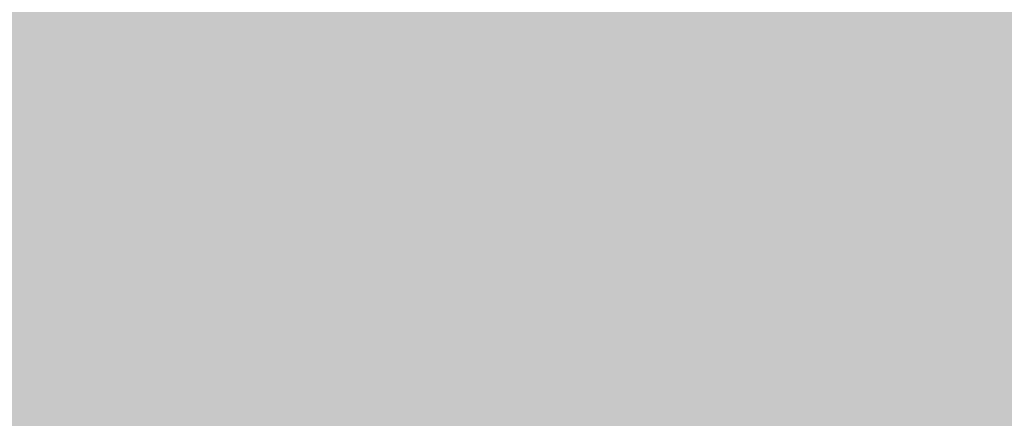
# Model space of a CAD drawing. Units: millimetres. Extents: x 0 to 2267, y 0 to 1823.
# Tile 127 of 256: x 1600.369 to 1605.705, y 1232.602 to 1234.764. Entities that reach past the tile are written whole.
import ezdxf

# ---------------------------------------------------------------- set-up
doc = ezdxf.new("R2010")
doc.units = ezdxf.units.MM
doc.header["$MEASUREMENT"] = 0
doc.layers.add('M-HATC', color=252, linetype='Continuous', lineweight=18)

msp = doc.modelspace()

# ---------------------------------------------------------------- hatches: boundary and pattern name
at = {"layer": 'M-HATC'}
h = msp.add_hatch(color=256, dxfattribs=at)
h.dxf.hatch_style = 1
h.paths.add_polyline_path([(2065.771, 1618.062, 0.236068), (2055.771, 1638.062), (1381.0868, 1638.062, 0.236068), (1371.0868, 1618.062), (1371.0868, 1603.062), (2055.771, 1603.062), (2065.771, 1603.062)])
h.paths.add_polyline_path([(2062.7718, 1550.2964), (2062.7718, 1560.2964), (1374.086, 1560.2964), (1374.086, 1550.2964), (1374.086, 1540.2964), (1384.086, 1540.2964), (1389.086, 1540.2964), (2062.7718, 1540.2964)])
h.paths.add_polyline_path([(1930.9289, 1282.7656), (1505.9289, 1282.7656), (1587.6276, 1235.5968, 0.131652), (1600.1276, 1232.2475), (1836.7302, 1232.2475, 0.131652), (1849.2302, 1235.5968)])
h.paths.add_polyline_path([(1930.9289, 1117.4171), (1905.9289, 1117.4171), (1505.9289, 1117.4171), (1505.9289, 1077.4171), (1930.9289, 1077.4171)])
h = msp.add_hatch(color=256, dxfattribs=at)
h.dxf.hatch_style = 1
h.paths.add_polyline_path([(2055.771, 1603.062), (1381.0868, 1603.062), (1381.0868, 1598.062), (2055.771, 1598.062)])
h.paths.add_polyline_path([(2055.771, 1598.062), (1381.0868, 1598.062), (1381.0868, 1593.062), (2055.771, 1593.062)])
h.paths.add_polyline_path([(2051.3074, 1536.7609), (1385.5504, 1536.7609), (1385.5504, 1526.7609), (1387.5504, 1526.7609), (1388.5366, 1525.0528), (1385.3319, 1521.2335), (1385.3319, 1521.2226), (2050.2542, 1522.7491), (2048.3212, 1525.0528), (2049.3074, 1526.7609), (2051.3074, 1526.7609)])
edge = h.paths.add_edge_path()
edge.add_arc((1847.5345, 1379.1492), 135, 222.603061, 222.890851, ccw=False)
edge.add_line((1748.1663, 1287.7656), (1683.0921, 1287.7656))
edge.add_arc((1583.7239, 1379.1492), 135, 317.109149, 317.396939, ccw=False)
edge.add_arc((1678.9686, 1290.6707), 5, 222.8909, 317.1091, ccw=False)
edge.add_arc((1774.2133, 1379.1492), 135, 222.603061, 222.890851, ccw=False)
edge.add_line((1674.8451, 1287.7656), (1609.7709, 1287.7656))
edge.add_arc((1510.4027, 1379.1492), 135, 317.109149, 317.396939, ccw=False)
edge.add_arc((1605.6474, 1290.6707), 5, 222.8909, 317.1091, ccw=False)
edge.add_arc((1700.8921, 1379.1492), 135, 222.603061, 222.890851, ccw=False)
edge.add_line((1601.5239, 1287.7656), (1536.4497, 1287.7656))
edge.add_arc((1437.0815, 1379.1492), 135, 317.109149, 317.396939, ccw=False)
edge.add_arc((1532.3262, 1290.6707), 5, 222.8909, 317.1091, ccw=False)
edge.add_arc((1627.5709, 1379.1492), 135, 222.603061, 222.890851, ccw=False)
edge.add_line((1528.2027, 1287.7656), (1505.9289, 1287.7656))
edge.add_spline(control_points=[(1505.9289, 1287.7656), (1504.2622, 1287.7656), (1504.2622, 1282.7656), (1505.9289, 1282.7656)], knot_values=[0, 0, 0, 0, 5, 5, 5, 5], degree=3, periodic=0)
edge.add_line((1505.9289, 1282.7656), (1930.9289, 1282.7656))
edge.add_spline(control_points=[(1930.9289, 1282.7656), (1932.5956, 1282.7656), (1932.5956, 1287.7656), (1930.9289, 1287.7656)], knot_values=[0, 0, 0, 0, 5, 5, 5, 5], degree=3, periodic=0)
edge.add_line((1930.9289, 1287.7656), (1903.0557, 1287.7656))
edge.add_arc((1803.6875, 1379.1492), 135, 317.109149, 317.396939, ccw=False)
edge.add_arc((1898.9322, 1290.6707), 5, 222.8909, 317.1091, ccw=False)
edge.add_arc((1994.1769, 1379.1492), 135, 222.603061, 222.890851, ccw=False)
edge.add_line((1894.8087, 1287.7656), (1829.7345, 1287.7656))
edge.add_arc((1730.3663, 1379.1492), 135, 317.109149, 317.396939, ccw=False)
edge.add_arc((1825.611, 1290.6707), 5, 222.8909, 317.1091, ccw=False)
edge.add_arc((1920.8557, 1379.1492), 135, 222.603061, 222.890851, ccw=False)
edge.add_line((1821.4875, 1287.7656), (1756.4133, 1287.7656))
edge.add_arc((1657.0451, 1379.1492), 135, 317.109149, 317.396939, ccw=False)
edge.add_arc((1752.2898, 1290.6707), 5, 222.8909, 317.1091, ccw=False)
edge = h.paths.add_edge_path()
edge.add_spline(control_points=[(1843.4289, 1227.2475), (1845.0956, 1227.2475), (1845.0956, 1232.2475), (1843.4289, 1232.2475)], knot_values=[0, 0, 0, 0, 5, 5, 5, 5], degree=3, periodic=0)
edge.add_line((1843.4289, 1232.2475), (1593.4289, 1232.2475))
edge.add_spline(control_points=[(1593.4289, 1232.2475), (1591.7622, 1232.2475), (1591.7622, 1227.2475), (1593.4289, 1227.2475)], knot_values=[0, 0, 0, 0, 5, 5, 5, 5], degree=3, periodic=0)
edge.add_line((1593.4289, 1227.2475), (1843.4289, 1227.2475))
h.paths.add_polyline_path([(1905.9289, 1127.4171), (1530.9289, 1127.4171, 0.414214), (1520.9289, 1117.4171), (1530.9289, 1117.4171), (1915.9289, 1117.4171, 0.414214)])
edge = h.paths.add_edge_path()
edge.add_arc((1397.0858, 1498.4078), 12.7299, 90.78215, 190.87871, ccw=False)
edge.add_line((1396.912, 1511.1365), (1428.0097, 1511.3488))
edge.add_line((1428.0097, 1511.3488), (1433.0097, 1511.3488))
edge.add_line((1433.0097, 1511.3488), (1434.439, 1511.3488))
edge.add_arc((1419.474, 1498.0804), 20, 41.561, 74.08211)
edge.add_line((1424.9592, 1517.3135), (1399.9351, 1517.2561))
edge.add_spline(control_points=[(1399.9307, 1517.2561), (1399.884, 1517.2131), (1399.8328, 1517.1689), (1399.7774, 1517.1236)], knot_values=[11.567499, 11.567499, 11.567499, 11.567499, 11.814249, 11.814249, 11.814249, 11.814249], degree=3, periodic=0)
edge.add_spline(control_points=[(1399.6328, 1517.0099), (1399.5831, 1516.9721), (1399.5307, 1516.9338), (1399.4759, 1516.8947)], knot_values=[11.167718, 11.167718, 11.167718, 11.167718, 11.365188, 11.365188, 11.365188, 11.365188], degree=3, periodic=0)
edge.add_spline(control_points=[(1399.3398, 1516.8001), (1399.1514, 1516.6719), (1398.9384, 1516.5377), (1398.704, 1516.3994)], knot_values=[10.376405, 10.376405, 10.376405, 10.376405, 11.00994, 11.00994, 11.00994, 11.00994], degree=3, periodic=0)
edge.add_spline(control_points=[(1398.6572, 1516.3719), (1398.5789, 1516.326), (1398.4983, 1516.2797), (1398.4155, 1516.2331)], knot_values=[10.125175, 10.125175, 10.125175, 10.125175, 10.334406, 10.334406, 10.334406, 10.334406], degree=3, periodic=0)
edge.add_spline(control_points=[(1398.2642, 1516.1487), (1398.196, 1516.1111), (1398.1263, 1516.0732), (1398.0555, 1516.0351)], knot_values=[9.832246, 9.832246, 9.832246, 9.832246, 9.999658, 9.999658, 9.999658, 9.999658], degree=3, periodic=0)
edge.add_spline(control_points=[(1397.9987, 1516.0048), (1397.7312, 1515.8621), (1397.446, 1515.7171), (1397.1466, 1515.5714)], knot_values=[9.161808, 9.161808, 9.161808, 9.161808, 9.787769, 9.787769, 9.787769, 9.787769], degree=3, periodic=0)
edge.add_spline(control_points=[(1397.1466, 1515.5714), (1396.8418, 1515.423), (1396.5222, 1515.274), (1396.1914, 1515.1262)], knot_values=[8.524455, 8.524455, 8.524455, 8.524455, 9.161808, 9.161808, 9.161808, 9.161808], degree=3, periodic=0)
edge.add_spline(control_points=[(1396.0777, 1515.0756), (1395.9854, 1515.0348), (1395.8922, 1514.994), (1395.7983, 1514.9534)], knot_values=[8.275193, 8.275193, 8.275193, 8.275193, 8.451726, 8.451726, 8.451726, 8.451726], degree=3, periodic=0)
edge.add_spline(control_points=[(1395.6018, 1514.8691), (1395.4997, 1514.8257), (1395.3968, 1514.7824), (1395.2932, 1514.7394)], knot_values=[7.962917, 7.962917, 7.962917, 7.962917, 8.152764, 8.152764, 8.152764, 8.152764], degree=3, periodic=0)
edge.add_spline(control_points=[(1395.2116, 1514.7057), (1394.8278, 1514.5475), (1394.4345, 1514.3929), (1394.0364, 1514.2442)], knot_values=[7.21254, 7.21254, 7.21254, 7.21254, 7.913148, 7.913148, 7.913148, 7.913148], degree=3, periodic=0)
edge.add_spline(control_points=[(1394.0364, 1514.2442), (1393.7076, 1514.1214), (1393.3754, 1514.0027), (1393.0427, 1513.8895)], knot_values=[6.633733, 6.633733, 6.633733, 6.633733, 7.21254, 7.21254, 7.21254, 7.21254], degree=3, periodic=0)
edge.add_spline(control_points=[(1392.8214, 1513.815), (1392.7198, 1513.7812), (1392.6181, 1513.7479), (1392.5166, 1513.7152)], knot_values=[6.328796, 6.328796, 6.328796, 6.328796, 6.505493, 6.505493, 6.505493, 6.505493], degree=3, periodic=0)
edge.add_spline(control_points=[(1392.5166, 1513.7152), (1392.3187, 1513.6515), (1392.1212, 1513.59), (1391.9244, 1513.531)], knot_values=[5.984605, 5.984605, 5.984605, 5.984605, 6.328796, 6.328796, 6.328796, 6.328796], degree=3, periodic=0)
edge.add_spline(control_points=[(1391.7915, 1513.4915), (1391.3122, 1513.3501), (1390.8384, 1513.2239), (1390.3784, 1513.1171)], knot_values=[5.066697, 5.066697, 5.066697, 5.066697, 5.907055, 5.907055, 5.907055, 5.907055], degree=3, periodic=0)
edge.add_spline(control_points=[(1390.3784, 1513.1171), (1390.1797, 1513.071), (1389.9836, 1513.0284), (1389.7907, 1512.9899)], knot_values=[4.70367, 4.70367, 4.70367, 4.70367, 5.066695, 5.066695, 5.066695, 5.066695], degree=3, periodic=0)
edge.add_spline(control_points=[(1389.422, 1512.9204), (1389.2459, 1512.8892), (1389.0729, 1512.8617), (1388.9036, 1512.8381)], knot_values=[4.130571, 4.130571, 4.130571, 4.130571, 4.469816, 4.469816, 4.469816, 4.469816], degree=3, periodic=0)
edge.add_spline(control_points=[(1388.9036, 1512.8381), (1388.591, 1512.7946), (1388.2911, 1512.7644), (1388.0071, 1512.7494)], knot_values=[3.504031, 3.504031, 3.504031, 3.504031, 4.130571, 4.130571, 4.130571, 4.130571], degree=3, periodic=0)
edge.add_spline(control_points=[(1387.9356, 1512.7459), (1387.8538, 1512.7423), (1387.7733, 1512.74), (1387.6944, 1512.739)], knot_values=[3.268866, 3.268866, 3.268866, 3.268866, 3.451164, 3.451164, 3.451164, 3.451164], degree=3, periodic=0)
edge.add_spline(control_points=[(1387.3351, 1512.7443), (1387.2076, 1512.7499), (1387.0847, 1512.7597), (1386.967, 1512.7739)], knot_values=[2.670686, 2.670686, 2.670686, 2.670686, 2.984, 2.984, 2.984, 2.984], degree=3, periodic=0)
edge.add_spline(control_points=[(1386.8327, 1512.7922), (1386.8209, 1512.7941), (1386.8092, 1512.7959), (1386.7975, 1512.7979)], knot_values=[2.516981, 2.516981, 2.516981, 2.516981, 2.549528, 2.549528, 2.549528, 2.549528], degree=3, periodic=0)
edge.add_spline(control_points=[(1386.4526, 1512.8735), (1386.4257, 1512.881), (1386.3993, 1512.889), (1386.3733, 1512.8972)], knot_values=[2.095869, 2.095869, 2.095869, 2.095869, 2.17941, 2.17941, 2.17941, 2.17941], degree=3, periodic=0)
edge.add_spline(control_points=[(1386.0691, 1513.0189), (1386.0634, 1513.0217), (1386.0577, 1513.0246), (1386.052, 1513.0275)], knot_values=[1.72453, 1.72453, 1.72453, 1.72453, 1.745933, 1.745933, 1.745933, 1.745933], degree=3, periodic=0)
edge.add_arc((1399.474, 1498.0804), 20, 131.82432, 180)
edge.add_arc((1630.3336, 1505.5484), 250.9708, 181.705176, 236.427975)
edge.add_arc((1605.3399, 1483.3044), 218.7822, 238.660829, 243.34961)
edge.add_arc((1647.0911, 1510.3592), 262.8986, 183.129836, 237.853442, ccw=False)
h.paths.add_polyline_path([(1406.5369, 1391.9644, 0.149382), (1491.5506, 1296.4418, -0.129517)], flags=17)
edge = h.paths.add_edge_path()
edge.add_arc((2037.3838, 1498.0804), 20, 0, 48.26587)
edge.add_spline(control_points=[(2050.6973, 1513.0052), (2050.6512, 1512.9847), (2050.6034, 1512.9655), (2050.5539, 1512.9477)], knot_values=[1.835652, 1.835652, 1.835652, 1.835652, 2.000781, 2.000781, 2.000781, 2.000781], degree=3, periodic=0)
edge.add_spline(control_points=[(2050.4616, 1512.9166), (2050.479, 1512.9221), (2050.4963, 1512.9277), (2050.5133, 1512.9335)], knot_values=[2.045477, 2.045477, 2.045477, 2.045477, 2.101389, 2.101389, 2.101389, 2.101389], degree=3, periodic=0)
edge.add_spline(control_points=[(2050.129, 1512.8342), (2050.1984, 1512.8473), (2050.2657, 1512.8623), (2050.3308, 1512.8792)], knot_values=[2.237629, 2.237629, 2.237629, 2.237629, 2.435841, 2.435841, 2.435841, 2.435841], degree=3, periodic=0)
edge.add_spline(control_points=[(2050.0946, 1512.8278), (2050.1061, 1512.8299), (2050.1176, 1512.832), (2050.129, 1512.8342)], knot_values=[2.435841, 2.435841, 2.435841, 2.435841, 2.468321, 2.468321, 2.468321, 2.468321], degree=3, periodic=0)
edge.add_spline(control_points=[(2049.7843, 1512.7851), (2049.8552, 1512.7922), (2049.9243, 1512.8008), (2049.9917, 1512.8109)], knot_values=[2.563852, 2.563852, 2.563852, 2.563852, 2.748541, 2.748541, 2.748541, 2.748541], degree=3, periodic=0)
edge.add_spline(control_points=[(2049.4052, 1512.7617), (2049.5364, 1512.7653), (2049.6629, 1512.773), (2049.7843, 1512.7851)], knot_values=[2.748541, 2.748541, 2.748541, 2.748541, 3.064882, 3.064882, 3.064882, 3.064882], degree=3, periodic=0)
edge.add_spline(control_points=[(2049.1698, 1512.7597), (2049.2336, 1512.7591), (2049.2965, 1512.7594), (2049.3584, 1512.7606)], knot_values=[3.102309, 3.102309, 3.102309, 3.102309, 3.2503, 3.2503, 3.2503, 3.2503], degree=3, periodic=0)
edge.add_spline(control_points=[(2048.8573, 1512.7691), (2048.9638, 1512.7638), (2049.068, 1512.7606), (2049.1698, 1512.7597)], knot_values=[3.2503, 3.2503, 3.2503, 3.2503, 3.486069, 3.486069, 3.486069, 3.486069], degree=3, periodic=0)
edge.add_spline(control_points=[(2048.6924, 1512.7789), (2048.3729, 1512.8009), (2048.0345, 1512.8411), (2047.6817, 1512.897)], knot_values=[3.606429, 3.606429, 3.606429, 3.606429, 4.2989, 4.2989, 4.2989, 4.2989], degree=3, periodic=0)
edge.add_spline(control_points=[(2047.6817, 1512.897), (2047.5458, 1512.9185), (2047.4077, 1512.9424), (2047.2678, 1512.9685)], knot_values=[4.2989, 4.2989, 4.2989, 4.2989, 4.565769, 4.565769, 4.565769, 4.565769], degree=3, periodic=0)
edge.add_spline(control_points=[(2047.2678, 1512.9685), (2047.1449, 1512.9914), (2047.0207, 1513.016), (2046.8951, 1513.0422)], knot_values=[4.565769, 4.565769, 4.565769, 4.565769, 4.799971, 4.799971, 4.799971, 4.799971], degree=3, periodic=0)
edge.add_spline(control_points=[(2046.8951, 1513.0422), (2046.5286, 1513.1188), (2046.1513, 1513.209), (2045.7676, 1513.3107)], knot_values=[4.799971, 4.799971, 4.799971, 4.799971, 5.483718, 5.483718, 5.483718, 5.483718], degree=3, periodic=0)
edge.add_spline(control_points=[(2045.7676, 1513.3107), (2045.3724, 1513.4154), (2044.9704, 1513.5322), (2044.5662, 1513.6588)], knot_values=[5.483718, 5.483718, 5.483718, 5.483718, 6.187866, 6.187866, 6.187866, 6.187866], degree=3, periodic=0)
edge.add_spline(control_points=[(2044.5662, 1513.6588), (2044.4149, 1513.7061), (2044.2633, 1513.7549), (2044.1116, 1513.8048)], knot_values=[6.187866, 6.187866, 6.187866, 6.187866, 6.451551, 6.451551, 6.451551, 6.451551], degree=3, periodic=0)
edge.add_spline(control_points=[(2044.1116, 1513.8048), (2043.9967, 1513.8427), (2043.8817, 1513.8813), (2043.7668, 1513.9205)], knot_values=[6.451551, 6.451551, 6.451551, 6.451551, 6.651434, 6.651434, 6.651434, 6.651434], degree=3, periodic=0)
edge.add_spline(control_points=[(2043.7668, 1513.9205), (2043.3716, 1514.0554), (2042.9774, 1514.1979), (2042.5886, 1514.3458)], knot_values=[6.651434, 6.651434, 6.651434, 6.651434, 7.338879, 7.338879, 7.338879, 7.338879], degree=3, periodic=0)
edge.add_spline(control_points=[(2042.5886, 1514.3458), (2042.1643, 1514.5071), (2041.7465, 1514.6749), (2041.3409, 1514.846)], knot_values=[7.338879, 7.338879, 7.338879, 7.338879, 8.089209, 8.089209, 8.089209, 8.089209], degree=3, periodic=0)
edge.add_spline(control_points=[(2041.3409, 1514.846), (2041.1028, 1514.9465), (2040.869, 1515.0481), (2040.6405, 1515.1502)], knot_values=[8.089209, 8.089209, 8.089209, 8.089209, 8.529587, 8.529587, 8.529587, 8.529587], degree=3, periodic=0)
edge.add_spline(control_points=[(2040.51, 1515.2089), (2040.0824, 1515.4022), (2039.6747, 1515.5971), (2039.295, 1515.7894)], knot_values=[8.613818, 8.613818, 8.613818, 8.613818, 9.44571, 9.44571, 9.44571, 9.44571], degree=3, periodic=0)
edge.add_spline(control_points=[(2039.295, 1515.7894), (2039.0618, 1515.9075), (2038.8391, 1516.0246), (2038.6288, 1516.1398)], knot_values=[9.44571, 9.44571, 9.44571, 9.44571, 9.956404, 9.956404, 9.956404, 9.956404], degree=3, periodic=0)
edge.add_spline(control_points=[(2038.6288, 1516.1398), (2038.5187, 1516.2001), (2038.4121, 1516.2598), (2038.309, 1516.3189)], knot_values=[9.956404, 9.956404, 9.956404, 9.956404, 10.223542, 10.223542, 10.223542, 10.223542], degree=3, periodic=0)
edge.add_spline(control_points=[(2038.309, 1516.3189), (2038.2138, 1516.3735), (2038.1216, 1516.4276), (2038.0328, 1516.481)], knot_values=[10.223542, 10.223542, 10.223542, 10.223542, 10.47051, 10.47051, 10.47051, 10.47051], degree=3, periodic=0)
edge.add_spline(control_points=[(2038.0328, 1516.481), (2037.7855, 1516.6296), (2037.5639, 1516.773), (2037.3722, 1516.909)], knot_values=[10.47051, 10.47051, 10.47051, 10.47051, 11.15767, 11.15767, 11.15767, 11.15767], degree=3, periodic=0)
edge.add_spline(control_points=[(2037.3722, 1516.909), (2037.2789, 1516.9752), (2037.1927, 1517.0396), (2037.1142, 1517.102)], knot_values=[11.15767, 11.15767, 11.15767, 11.15767, 11.49227, 11.49227, 11.49227, 11.49227], degree=3, periodic=0)
edge.add_spline(control_points=[(2036.8564, 1517.3259), (2036.9148, 1517.2692), (2036.9814, 1517.2103), (2037.0557, 1517.1492)], knot_values=[11.577341, 11.577341, 11.577341, 11.577341, 11.91035, 11.91035, 11.91035, 11.91035], degree=3, periodic=0)
edge.add_spline(control_points=[(2036.8074, 1517.3748), (2036.823, 1517.3587), (2036.8393, 1517.3424), (2036.8564, 1517.3259)], knot_values=[11.91035, 11.91035, 11.91035, 11.91035, 12.007402, 12.007402, 12.007402, 12.007402], degree=3, periodic=0)
edge.add_spline(control_points=[(2036.7017, 1517.494), (2036.7104, 1517.483), (2036.7196, 1517.4719), (2036.7291, 1517.4606)], knot_values=[12.184155, 12.184155, 12.184155, 12.184155, 12.255409, 12.255409, 12.255409, 12.255409], degree=3, periodic=0)
edge.add_spline(control_points=[(2036.6159, 1517.6205), (2036.62, 1517.613), (2036.6243, 1517.6055), (2036.6289, 1517.5979)], knot_values=[12.487913, 12.487913, 12.487913, 12.487913, 12.541035, 12.541035, 12.541035, 12.541035], degree=3, periodic=0)
edge.add_spline(control_points=[(2036.5635, 1517.786), (2036.5637, 1517.7794), (2036.5642, 1517.7726), (2036.565, 1517.7658)], knot_values=[12.911761, 12.911761, 12.911761, 12.911761, 12.968286, 12.968286, 12.968286, 12.968286], degree=3, periodic=0)
edge.add_spline(control_points=[(2036.6166, 1517.9304), (2036.6125, 1517.9259), (2036.6086, 1517.9212), (2036.6049, 1517.9165)], knot_values=[13.382527, 13.382527, 13.382527, 13.382527, 13.433791, 13.433791, 13.433791, 13.433791], degree=3, periodic=0)
edge.add_spline(control_points=[(2036.749, 1518.017), (2036.7361, 1518.0116), (2036.7239, 1518.006), (2036.7124, 1518.0002)], knot_values=[13.726299, 13.726299, 13.726299, 13.726299, 13.809928, 13.809928, 13.809928, 13.809928], degree=3, periodic=0)
edge.add_spline(control_points=[(2036.8604, 1518.0528), (2036.8386, 1518.0474), (2036.8181, 1518.0416), (2036.7988, 1518.0353)], knot_values=[13.910887, 13.910887, 13.910887, 13.910887, 14.02153, 14.02153, 14.02153, 14.02153], degree=3, periodic=0)
edge.add_line((2036.9639, 1518.0804), (2032.3838, 1518.0804))
edge.add_line((2032.3838, 1518.0804), (2027.3838, 1518.0804))
edge.add_line((2027.3838, 1518.0804), (2022.3838, 1518.0804))
edge.add_line((2022.3838, 1518.0804), (2017.3838, 1518.0804))
edge.add_arc((2017.3838, 1498.0804), 20, 90, 138.439)
edge.add_line((2002.4188, 1511.3488), (2003.8481, 1511.3488))
edge.add_line((2003.8481, 1511.3488), (2008.8481, 1511.3488))
edge.add_line((2008.8481, 1511.3488), (2039.772, 1511.1377))
edge.add_arc((2039.772, 1498.4078), 12.7299, -10.87871, 90, ccw=False)
edge.add_arc((1789.7668, 1510.3592), 262.8986, 302.146558, 356.870164, ccw=False)
edge.add_arc((1831.5179, 1483.3044), 218.7822, 296.65039, 301.339171)
edge.add_arc((1806.5242, 1505.5484), 250.9708, 303.572025, 358.294824)
h.paths.add_polyline_path([(2030.321, 1391.9644, -0.129517), (1945.3072, 1296.4418, 0.149382)], flags=17)
edge = h.paths.add_edge_path()
edge.add_spline(control_points=[(2037.2464, 1518.0821), (2037.2898, 1518.081), (2037.3355, 1518.0804), (2037.3838, 1518.0804)], knot_values=[0.000012, 0.000012, 0.000012, 0.000012, 0.144754, 0.144754, 0.144754, 0.144754], degree=3, periodic=0)
edge.add_line((2037.3357, 1518.0804), (2037.0096, 1518.0804))
edge.add_spline(control_points=[(2037.0096, 1518.0804), (2036.9822, 1518.0768), (2036.956, 1518.0727), (2036.9312, 1518.0681)], knot_values=[14.13465, 14.13465, 14.13465, 14.13465, 14.247197, 14.247197, 14.247197, 14.247197], degree=3, periodic=0)
edge.add_spline(control_points=[(2036.9312, 1518.0681), (2036.9276, 1518.0674), (2036.9241, 1518.0667), (2036.9205, 1518.0661)], knot_values=[14.118315, 14.118315, 14.118315, 14.118315, 14.13465, 14.13465, 14.13465, 14.13465], degree=3, periodic=0)
edge.add_spline(control_points=[(2036.9205, 1518.0661), (2036.9118, 1518.0644), (2036.9032, 1518.0626), (2036.8948, 1518.0608)], knot_values=[14.078086, 14.078086, 14.078086, 14.078086, 14.118315, 14.118315, 14.118315, 14.118315], degree=3, periodic=0)
edge.add_spline(control_points=[(2036.8948, 1518.0608), (2036.883, 1518.0583), (2036.8716, 1518.0556), (2036.8604, 1518.0528)], knot_values=[14.02153, 14.02153, 14.02153, 14.02153, 14.078086, 14.078086, 14.078086, 14.078086], degree=3, periodic=0)
edge.add_spline(control_points=[(2036.8604, 1518.0528), (2036.8386, 1518.0474), (2036.8181, 1518.0416), (2036.7988, 1518.0353)], knot_values=[13.910887, 13.910887, 13.910887, 13.910887, 14.02153, 14.02153, 14.02153, 14.02153], degree=3, periodic=0)
edge.add_spline(control_points=[(2036.7988, 1518.0353), (2036.7981, 1518.035), (2036.7974, 1518.0348), (2036.7967, 1518.0346)], knot_values=[13.906906, 13.906906, 13.906906, 13.906906, 13.910887, 13.910887, 13.910887, 13.910887], degree=3, periodic=0)
edge.add_spline(control_points=[(2036.7967, 1518.0346), (2036.7882, 1518.0318), (2036.7799, 1518.0289), (2036.7719, 1518.0259)], knot_values=[13.857826, 13.857826, 13.857826, 13.857826, 13.906906, 13.906906, 13.906906, 13.906906], degree=3, periodic=0)
edge.add_spline(control_points=[(2036.7719, 1518.0259), (2036.764, 1518.023), (2036.7564, 1518.02), (2036.749, 1518.017)], knot_values=[13.809928, 13.809928, 13.809928, 13.809928, 13.857826, 13.857826, 13.857826, 13.857826], degree=3, periodic=0)
edge.add_spline(control_points=[(2036.749, 1518.017), (2036.7361, 1518.0116), (2036.7239, 1518.006), (2036.7124, 1518.0002)], knot_values=[13.726299, 13.726299, 13.726299, 13.726299, 13.809928, 13.809928, 13.809928, 13.809928], degree=3, periodic=0)
edge.add_spline(control_points=[(2036.7124, 1518.0002), (2036.7121, 1518), (2036.7118, 1517.9999), (2036.7115, 1517.9997)], knot_values=[13.723993, 13.723993, 13.723993, 13.723993, 13.726299, 13.726299, 13.726299, 13.726299], degree=3, periodic=0)
edge.add_spline(control_points=[(2036.7115, 1517.9997), (2036.7063, 1517.9971), (2036.7013, 1517.9944), (2036.6965, 1517.9917)], knot_values=[13.686536, 13.686536, 13.686536, 13.686536, 13.723993, 13.723993, 13.723993, 13.723993], degree=3, periodic=0)
edge.add_spline(control_points=[(2036.6965, 1517.9917), (2036.6919, 1517.9891), (2036.6874, 1517.9865), (2036.6831, 1517.9839)], knot_values=[13.651251, 13.651251, 13.651251, 13.651251, 13.686536, 13.686536, 13.686536, 13.686536], degree=3, periodic=0)
edge.add_spline(control_points=[(2036.6831, 1517.9839), (2036.6764, 1517.9798), (2036.67, 1517.9757), (2036.6639, 1517.9714)], knot_values=[13.596804, 13.596804, 13.596804, 13.596804, 13.651251, 13.651251, 13.651251, 13.651251], degree=3, periodic=0)
edge.add_spline(control_points=[(2036.6639, 1517.9714), (2036.6636, 1517.9712), (2036.6633, 1517.9709), (2036.6629, 1517.9707)], knot_values=[13.593956, 13.593956, 13.593956, 13.593956, 13.596804, 13.596804, 13.596804, 13.596804], degree=3, periodic=0)
edge.add_spline(control_points=[(2036.6629, 1517.9707), (2036.6603, 1517.9689), (2036.6577, 1517.967), (2036.6552, 1517.9651)], knot_values=[13.570322, 13.570322, 13.570322, 13.570322, 13.593956, 13.593956, 13.593956, 13.593956], degree=3, periodic=0)
edge.add_spline(control_points=[(2036.6552, 1517.9651), (2036.6525, 1517.9631), (2036.6499, 1517.9611), (2036.6474, 1517.9591)], knot_values=[13.545477, 13.545477, 13.545477, 13.545477, 13.570322, 13.570322, 13.570322, 13.570322], degree=3, periodic=0)
edge.add_spline(control_points=[(2036.6474, 1517.9591), (2036.6472, 1517.9589), (2036.6471, 1517.9588), (2036.6469, 1517.9587)], knot_values=[13.543931, 13.543931, 13.543931, 13.543931, 13.545477, 13.545477, 13.545477, 13.545477], degree=3, periodic=0)
edge.add_spline(control_points=[(2036.6469, 1517.9587), (2036.6412, 1517.9541), (2036.6358, 1517.9494), (2036.6307, 1517.9447)], knot_values=[13.488237, 13.488237, 13.488237, 13.488237, 13.543931, 13.543931, 13.543931, 13.543931], degree=3, periodic=0)
edge.add_spline(control_points=[(2036.6307, 1517.9447), (2036.6282, 1517.9423), (2036.6257, 1517.9399), (2036.6233, 1517.9374)], knot_values=[13.460307, 13.460307, 13.460307, 13.460307, 13.488237, 13.488237, 13.488237, 13.488237], degree=3, periodic=0)
edge.add_spline(control_points=[(2036.6233, 1517.9374), (2036.6215, 1517.9356), (2036.6198, 1517.9338), (2036.6181, 1517.932)], knot_values=[13.439712, 13.439712, 13.439712, 13.439712, 13.460307, 13.460307, 13.460307, 13.460307], degree=3, periodic=0)
edge.add_spline(control_points=[(2036.6181, 1517.932), (2036.6176, 1517.9315), (2036.6171, 1517.9309), (2036.6166, 1517.9304)], knot_values=[13.433791, 13.433791, 13.433791, 13.433791, 13.439712, 13.439712, 13.439712, 13.439712], degree=3, periodic=0)
edge.add_spline(control_points=[(2036.6166, 1517.9304), (2036.6125, 1517.9259), (2036.6086, 1517.9212), (2036.6049, 1517.9165)], knot_values=[13.382527, 13.382527, 13.382527, 13.382527, 13.433791, 13.433791, 13.433791, 13.433791], degree=3, periodic=0)
edge.add_spline(control_points=[(2036.6049, 1517.9165), (2036.6026, 1517.9135), (2036.6004, 1517.9104), (2036.5982, 1517.9074)], knot_values=[13.350017, 13.350017, 13.350017, 13.350017, 13.382527, 13.382527, 13.382527, 13.382527], degree=3, periodic=0)
edge.add_spline(control_points=[(2036.5982, 1517.9074), (2036.5972, 1517.9059), (2036.5962, 1517.9043), (2036.5952, 1517.9028)], knot_values=[13.333922, 13.333922, 13.333922, 13.333922, 13.350017, 13.350017, 13.350017, 13.350017], degree=3, periodic=0)
edge.add_spline(control_points=[(2036.5952, 1517.9028), (2036.5945, 1517.9018), (2036.5939, 1517.9009), (2036.5933, 1517.8999)], knot_values=[13.323828, 13.323828, 13.323828, 13.323828, 13.333922, 13.333922, 13.333922, 13.333922], degree=3, periodic=0)
edge.add_spline(control_points=[(2036.5933, 1517.8999), (2036.5905, 1517.8955), (2036.5879, 1517.8909), (2036.5855, 1517.8864)], knot_values=[13.277545, 13.277545, 13.277545, 13.277545, 13.323828, 13.323828, 13.323828, 13.323828], degree=3, periodic=0)
edge.add_spline(control_points=[(2036.5855, 1517.8864), (2036.5836, 1517.8827), (2036.5817, 1517.8789), (2036.5801, 1517.8751)], knot_values=[13.240119, 13.240119, 13.240119, 13.240119, 13.277545, 13.277545, 13.277545, 13.277545], degree=3, periodic=0)
edge.add_spline(control_points=[(2036.5801, 1517.8751), (2036.5795, 1517.8739), (2036.579, 1517.8727), (2036.5785, 1517.8715)], knot_values=[13.228211, 13.228211, 13.228211, 13.228211, 13.240119, 13.240119, 13.240119, 13.240119], degree=3, periodic=0)
edge.add_spline(control_points=[(2036.5785, 1517.8715), (2036.578, 1517.8702), (2036.5774, 1517.869), (2036.5769, 1517.8677)], knot_values=[13.215717, 13.215717, 13.215717, 13.215717, 13.228211, 13.228211, 13.228211, 13.228211], degree=3, periodic=0)
edge.add_spline(control_points=[(2036.5769, 1517.8677), (2036.5755, 1517.864), (2036.5741, 1517.8603), (2036.5729, 1517.8565)], knot_values=[13.179847, 13.179847, 13.179847, 13.179847, 13.215717, 13.215717, 13.215717, 13.215717], degree=3, periodic=0)
edge.add_spline(control_points=[(2036.5729, 1517.8565), (2036.5713, 1517.8515), (2036.5699, 1517.8464), (2036.5687, 1517.8413)], knot_values=[13.132017, 13.132017, 13.132017, 13.132017, 13.179847, 13.179847, 13.179847, 13.179847], degree=3, periodic=0)
edge.add_spline(control_points=[(2036.5687, 1517.8413), (2036.5684, 1517.8402), (2036.5682, 1517.8392), (2036.568, 1517.8382)], knot_values=[13.122482, 13.122482, 13.122482, 13.122482, 13.132017, 13.132017, 13.132017, 13.132017], degree=3, periodic=0)
edge.add_spline(control_points=[(2036.568, 1517.8382), (2036.5676, 1517.8363), (2036.5672, 1517.8345), (2036.5669, 1517.8327)], knot_values=[13.105592, 13.105592, 13.105592, 13.105592, 13.122482, 13.122482, 13.122482, 13.122482], degree=3, periodic=0)
edge.add_spline(control_points=[(2036.5669, 1517.8327), (2036.5662, 1517.8292), (2036.5657, 1517.8257), (2036.5652, 1517.8222)], knot_values=[13.074063, 13.074063, 13.074063, 13.074063, 13.105592, 13.105592, 13.105592, 13.105592], degree=3, periodic=0)
edge.add_spline(control_points=[(2036.5652, 1517.8222), (2036.5652, 1517.8222), (2036.5652, 1517.8222), (2036.5652, 1517.8222)], knot_values=[13.074043, 13.074043, 13.074043, 13.074043, 13.074063, 13.074063, 13.074063, 13.074063], degree=3, periodic=0)
edge.add_spline(control_points=[(2036.5652, 1517.8222), (2036.5644, 1517.8164), (2036.5639, 1517.8106), (2036.5636, 1517.8046)], knot_values=[13.021884, 13.021884, 13.021884, 13.021884, 13.074043, 13.074043, 13.074043, 13.074043], degree=3, periodic=0)
edge.add_spline(control_points=[(2036.5636, 1517.8046), (2036.5636, 1517.804), (2036.5636, 1517.8034), (2036.5635, 1517.8028)], knot_values=[13.01674, 13.01674, 13.01674, 13.01674, 13.021884, 13.021884, 13.021884, 13.021884], degree=3, periodic=0)
edge.add_spline(control_points=[(2036.5635, 1517.8028), (2036.5634, 1517.8005), (2036.5634, 1517.7982), (2036.5634, 1517.7958)], knot_values=[12.996438, 12.996438, 12.996438, 12.996438, 13.01674, 13.01674, 13.01674, 13.01674], degree=3, periodic=0)
edge.add_spline(control_points=[(2036.5634, 1517.7958), (2036.5633, 1517.7926), (2036.5634, 1517.7893), (2036.5635, 1517.786)], knot_values=[12.968286, 12.968286, 12.968286, 12.968286, 12.996438, 12.996438, 12.996438, 12.996438], degree=3, periodic=0)
edge.add_spline(control_points=[(2036.5635, 1517.786), (2036.5637, 1517.7794), (2036.5642, 1517.7726), (2036.565, 1517.7658)], knot_values=[12.911761, 12.911761, 12.911761, 12.911761, 12.968286, 12.968286, 12.968286, 12.968286], degree=3, periodic=0)
edge.add_spline(control_points=[(2036.565, 1517.7658), (2036.565, 1517.7657), (2036.565, 1517.7656), (2036.565, 1517.7656)], knot_values=[12.911017, 12.911017, 12.911017, 12.911017, 12.911761, 12.911761, 12.911761, 12.911761], degree=3, periodic=0)
edge.add_spline(control_points=[(2036.565, 1517.7656), (2036.5654, 1517.7625), (2036.5658, 1517.7593), (2036.5663, 1517.7562)], knot_values=[12.88528, 12.88528, 12.88528, 12.88528, 12.911017, 12.911017, 12.911017, 12.911017], degree=3, periodic=0)
edge.add_spline(control_points=[(2036.5663, 1517.7562), (2036.5667, 1517.7534), (2036.5672, 1517.7506), (2036.5677, 1517.7478)], knot_values=[12.862519, 12.862519, 12.862519, 12.862519, 12.88528, 12.88528, 12.88528, 12.88528], degree=3, periodic=0)
edge.add_spline(control_points=[(2036.5677, 1517.7478), (2036.5678, 1517.7474), (2036.5679, 1517.7469), (2036.568, 1517.7465)], knot_values=[12.858885, 12.858885, 12.858885, 12.858885, 12.862519, 12.862519, 12.862519, 12.862519], degree=3, periodic=0)
edge.add_spline(control_points=[(2036.568, 1517.7465), (2036.5692, 1517.7399), (2036.5707, 1517.7332), (2036.5724, 1517.7264)], knot_values=[12.8053, 12.8053, 12.8053, 12.8053, 12.858885, 12.858885, 12.858885, 12.858885], degree=3, periodic=0)
edge.add_spline(control_points=[(2036.5724, 1517.7264), (2036.5734, 1517.7226), (2036.5745, 1517.7187), (2036.5756, 1517.7149)], knot_values=[12.775176, 12.775176, 12.775176, 12.775176, 12.8053, 12.8053, 12.8053, 12.8053], degree=3, periodic=0)
edge.add_spline(control_points=[(2036.5756, 1517.7149), (2036.5763, 1517.7125), (2036.577, 1517.7102), (2036.5778, 1517.7078)], knot_values=[12.756759, 12.756759, 12.756759, 12.756759, 12.775176, 12.775176, 12.775176, 12.775176], degree=3, periodic=0)
edge.add_spline(control_points=[(2036.5778, 1517.7078), (2036.5781, 1517.7067), (2036.5784, 1517.7057), (2036.5787, 1517.7047)], knot_values=[12.748742, 12.748742, 12.748742, 12.748742, 12.756759, 12.756759, 12.756759, 12.756759], degree=3, periodic=0)
edge.add_spline(control_points=[(2036.5787, 1517.7047), (2036.5808, 1517.6983), (2036.5831, 1517.6919), (2036.5856, 1517.6854)], knot_values=[12.69959, 12.69959, 12.69959, 12.69959, 12.748742, 12.748742, 12.748742, 12.748742], degree=3, periodic=0)
edge.add_spline(control_points=[(2036.5856, 1517.6854), (2036.5876, 1517.68), (2036.5898, 1517.6746), (2036.5921, 1517.6692)], knot_values=[12.659038, 12.659038, 12.659038, 12.659038, 12.69959, 12.69959, 12.69959, 12.69959], degree=3, periodic=0)
edge.add_spline(control_points=[(2036.5921, 1517.6692), (2036.594, 1517.6648), (2036.5959, 1517.6605), (2036.5979, 1517.6561)], knot_values=[12.626806, 12.626806, 12.626806, 12.626806, 12.659038, 12.659038, 12.659038, 12.659038], degree=3, periodic=0)
edge.add_spline(control_points=[(2036.5979, 1517.6561), (2036.5984, 1517.6551), (2036.5989, 1517.6541), (2036.5993, 1517.6531)], knot_values=[12.619394, 12.619394, 12.619394, 12.619394, 12.626806, 12.626806, 12.626806, 12.626806], degree=3, periodic=0)
edge.add_spline(control_points=[(2036.5993, 1517.6531), (2036.6043, 1517.6424), (2036.6099, 1517.6315), (2036.6159, 1517.6205)], knot_values=[12.541039, 12.541039, 12.541039, 12.541039, 12.619394, 12.619394, 12.619394, 12.619394], degree=3, periodic=0)
edge.add_spline(control_points=[(2036.6159, 1517.6205), (2036.6159, 1517.6205), (2036.6159, 1517.6205), (2036.6159, 1517.6205)], knot_values=[12.541035, 12.541035, 12.541035, 12.541035, 12.541039, 12.541039, 12.541039, 12.541039], degree=3, periodic=0)
edge.add_spline(control_points=[(2036.6159, 1517.6205), (2036.62, 1517.613), (2036.6243, 1517.6055), (2036.6289, 1517.5979)], knot_values=[12.487913, 12.487913, 12.487913, 12.487913, 12.541035, 12.541035, 12.541035, 12.541035], degree=3, periodic=0)
edge.add_spline(control_points=[(2036.6289, 1517.5979), (2036.6326, 1517.5916), (2036.6365, 1517.5853), (2036.6406, 1517.5789)], knot_values=[12.443982, 12.443982, 12.443982, 12.443982, 12.487913, 12.487913, 12.487913, 12.487913], degree=3, periodic=0)
edge.add_spline(control_points=[(2036.6406, 1517.5789), (2036.6414, 1517.5776), (2036.6423, 1517.5763), (2036.6431, 1517.5749)], knot_values=[12.434996, 12.434996, 12.434996, 12.434996, 12.443982, 12.443982, 12.443982, 12.443982], degree=3, periodic=0)
edge.add_spline(control_points=[(2036.6431, 1517.5749), (2036.6531, 1517.5596), (2036.6639, 1517.5439), (2036.6756, 1517.528)], knot_values=[12.329647, 12.329647, 12.329647, 12.329647, 12.434996, 12.434996, 12.434996, 12.434996], degree=3, periodic=0)
edge.add_spline(control_points=[(2036.6756, 1517.528), (2036.6839, 1517.5168), (2036.6925, 1517.5055), (2036.7017, 1517.494)], knot_values=[12.255409, 12.255409, 12.255409, 12.255409, 12.329647, 12.329647, 12.329647, 12.329647], degree=3, periodic=0)
edge.add_spline(control_points=[(2036.7017, 1517.494), (2036.7104, 1517.483), (2036.7196, 1517.4719), (2036.7291, 1517.4606)], knot_values=[12.184155, 12.184155, 12.184155, 12.184155, 12.255409, 12.255409, 12.255409, 12.255409], degree=3, periodic=0)
edge.add_spline(control_points=[(2036.7291, 1517.4606), (2036.7436, 1517.4435), (2036.759, 1517.4262), (2036.7753, 1517.4085)], knot_values=[12.075961, 12.075961, 12.075961, 12.075961, 12.184155, 12.184155, 12.184155, 12.184155], degree=3, periodic=0)
edge.add_spline(control_points=[(2036.7753, 1517.4085), (2036.7763, 1517.4075), (2036.7773, 1517.4064), (2036.7783, 1517.4054)], knot_values=[12.069502, 12.069502, 12.069502, 12.069502, 12.075961, 12.075961, 12.075961, 12.075961], degree=3, periodic=0)
edge.add_spline(control_points=[(2036.7783, 1517.4054), (2036.7877, 1517.3953), (2036.7974, 1517.385), (2036.8074, 1517.3748)], knot_values=[12.007402, 12.007402, 12.007402, 12.007402, 12.069502, 12.069502, 12.069502, 12.069502], degree=3, periodic=0)
edge.add_spline(control_points=[(2036.8074, 1517.3748), (2036.823, 1517.3587), (2036.8393, 1517.3424), (2036.8564, 1517.3259)], knot_values=[11.91035, 11.91035, 11.91035, 11.91035, 12.007402, 12.007402, 12.007402, 12.007402], degree=3, periodic=0)
edge.add_spline(control_points=[(2036.8564, 1517.3259), (2036.9148, 1517.2692), (2036.9814, 1517.2103), (2037.0557, 1517.1492)], knot_values=[11.577341, 11.577341, 11.577341, 11.577341, 11.91035, 11.91035, 11.91035, 11.91035], degree=3, periodic=0)
edge.add_spline(control_points=[(2037.0557, 1517.1492), (2037.0747, 1517.1336), (2037.0942, 1517.1179), (2037.1142, 1517.102)], knot_values=[11.49227, 11.49227, 11.49227, 11.49227, 11.577341, 11.577341, 11.577341, 11.577341], degree=3, periodic=0)
edge.add_spline(control_points=[(2037.1142, 1517.102), (2037.1927, 1517.0396), (2037.2789, 1516.9752), (2037.3722, 1516.909)], knot_values=[11.15767, 11.15767, 11.15767, 11.15767, 11.49227, 11.49227, 11.49227, 11.49227], degree=3, periodic=0)
edge.add_spline(control_points=[(2037.3722, 1516.909), (2037.5639, 1516.773), (2037.7855, 1516.6296), (2038.0328, 1516.481)], knot_values=[10.47051, 10.47051, 10.47051, 10.47051, 11.15767, 11.15767, 11.15767, 11.15767], degree=3, periodic=0)
edge.add_spline(control_points=[(2038.0328, 1516.481), (2038.1216, 1516.4276), (2038.2138, 1516.3735), (2038.309, 1516.3189)], knot_values=[10.223542, 10.223542, 10.223542, 10.223542, 10.47051, 10.47051, 10.47051, 10.47051], degree=3, periodic=0)
edge.add_spline(control_points=[(2038.309, 1516.3189), (2038.4121, 1516.2598), (2038.5187, 1516.2001), (2038.6288, 1516.1398)], knot_values=[9.956404, 9.956404, 9.956404, 9.956404, 10.223542, 10.223542, 10.223542, 10.223542], degree=3, periodic=0)
edge.add_spline(control_points=[(2038.6288, 1516.1398), (2038.8391, 1516.0246), (2039.0618, 1515.9075), (2039.295, 1515.7894)], knot_values=[9.44571, 9.44571, 9.44571, 9.44571, 9.956404, 9.956404, 9.956404, 9.956404], degree=3, periodic=0)
edge.add_spline(control_points=[(2039.295, 1515.7894), (2039.6747, 1515.5971), (2040.0824, 1515.4022), (2040.51, 1515.2089)], knot_values=[8.613818, 8.613818, 8.613818, 8.613818, 9.44571, 9.44571, 9.44571, 9.44571], degree=3, periodic=0)
edge.add_spline(control_points=[(2040.51, 1515.2089), (2040.5533, 1515.1893), (2040.5968, 1515.1697), (2040.6405, 1515.1502)], knot_values=[8.529587, 8.529587, 8.529587, 8.529587, 8.613818, 8.613818, 8.613818, 8.613818], degree=3, periodic=0)
edge.add_spline(control_points=[(2040.6405, 1515.1502), (2040.869, 1515.0481), (2041.1028, 1514.9465), (2041.3409, 1514.846)], knot_values=[8.089209, 8.089209, 8.089209, 8.089209, 8.529587, 8.529587, 8.529587, 8.529587], degree=3, periodic=0)
edge.add_spline(control_points=[(2041.3409, 1514.846), (2041.7465, 1514.6749), (2042.1643, 1514.5071), (2042.5886, 1514.3458)], knot_values=[7.338879, 7.338879, 7.338879, 7.338879, 8.089209, 8.089209, 8.089209, 8.089209], degree=3, periodic=0)
edge.add_spline(control_points=[(2042.5886, 1514.3458), (2042.9774, 1514.1979), (2043.3716, 1514.0554), (2043.7668, 1513.9205)], knot_values=[6.651434, 6.651434, 6.651434, 6.651434, 7.338879, 7.338879, 7.338879, 7.338879], degree=3, periodic=0)
edge.add_spline(control_points=[(2043.7668, 1513.9205), (2043.8817, 1513.8813), (2043.9967, 1513.8427), (2044.1116, 1513.8048)], knot_values=[6.451551, 6.451551, 6.451551, 6.451551, 6.651434, 6.651434, 6.651434, 6.651434], degree=3, periodic=0)
edge.add_spline(control_points=[(2044.1116, 1513.8048), (2044.2633, 1513.7549), (2044.4149, 1513.7061), (2044.5662, 1513.6588)], knot_values=[6.187866, 6.187866, 6.187866, 6.187866, 6.451551, 6.451551, 6.451551, 6.451551], degree=3, periodic=0)
edge.add_spline(control_points=[(2044.5662, 1513.6588), (2044.9704, 1513.5322), (2045.3724, 1513.4154), (2045.7676, 1513.3107)], knot_values=[5.483718, 5.483718, 5.483718, 5.483718, 6.187866, 6.187866, 6.187866, 6.187866], degree=3, periodic=0)
edge.add_spline(control_points=[(2045.7676, 1513.3107), (2046.1513, 1513.209), (2046.5286, 1513.1188), (2046.8951, 1513.0422)], knot_values=[4.799971, 4.799971, 4.799971, 4.799971, 5.483718, 5.483718, 5.483718, 5.483718], degree=3, periodic=0)
edge.add_spline(control_points=[(2046.8951, 1513.0422), (2047.0207, 1513.016), (2047.1449, 1512.9914), (2047.2678, 1512.9685)], knot_values=[4.565769, 4.565769, 4.565769, 4.565769, 4.799971, 4.799971, 4.799971, 4.799971], degree=3, periodic=0)
edge.add_spline(control_points=[(2047.2678, 1512.9685), (2047.4077, 1512.9424), (2047.5458, 1512.9185), (2047.6817, 1512.897)], knot_values=[4.2989, 4.2989, 4.2989, 4.2989, 4.565769, 4.565769, 4.565769, 4.565769], degree=3, periodic=0)
edge.add_spline(control_points=[(2047.6817, 1512.897), (2048.0345, 1512.8411), (2048.3729, 1512.8009), (2048.6924, 1512.7789)], knot_values=[3.606429, 3.606429, 3.606429, 3.606429, 4.2989, 4.2989, 4.2989, 4.2989], degree=3, periodic=0)
edge.add_spline(control_points=[(2048.6924, 1512.7789), (2048.7479, 1512.7751), (2048.8029, 1512.7718), (2048.8573, 1512.7691)], knot_values=[3.486069, 3.486069, 3.486069, 3.486069, 3.606429, 3.606429, 3.606429, 3.606429], degree=3, periodic=0)
edge.add_spline(control_points=[(2048.8573, 1512.7691), (2048.9638, 1512.7638), (2049.068, 1512.7606), (2049.1698, 1512.7597)], knot_values=[3.2503, 3.2503, 3.2503, 3.2503, 3.486069, 3.486069, 3.486069, 3.486069], degree=3, periodic=0)
edge.add_spline(control_points=[(2049.1698, 1512.7597), (2049.2336, 1512.7591), (2049.2965, 1512.7594), (2049.3584, 1512.7606)], knot_values=[3.102309, 3.102309, 3.102309, 3.102309, 3.2503, 3.2503, 3.2503, 3.2503], degree=3, periodic=0)
edge.add_spline(control_points=[(2049.3584, 1512.7606), (2049.3741, 1512.7609), (2049.3897, 1512.7613), (2049.4052, 1512.7617)], knot_values=[3.064882, 3.064882, 3.064882, 3.064882, 3.102309, 3.102309, 3.102309, 3.102309], degree=3, periodic=0)
edge.add_spline(control_points=[(2049.4052, 1512.7617), (2049.5364, 1512.7653), (2049.6629, 1512.773), (2049.7843, 1512.7851)], knot_values=[2.748541, 2.748541, 2.748541, 2.748541, 3.064882, 3.064882, 3.064882, 3.064882], degree=3, periodic=0)
edge.add_spline(control_points=[(2049.7843, 1512.7851), (2049.8552, 1512.7922), (2049.9243, 1512.8008), (2049.9917, 1512.8109)], knot_values=[2.563852, 2.563852, 2.563852, 2.563852, 2.748541, 2.748541, 2.748541, 2.748541], degree=3, periodic=0)
edge.add_spline(control_points=[(2049.9917, 1512.8109), (2050.0265, 1512.8161), (2050.0608, 1512.8218), (2050.0946, 1512.8278)], knot_values=[2.468321, 2.468321, 2.468321, 2.468321, 2.563852, 2.563852, 2.563852, 2.563852], degree=3, periodic=0)
edge.add_spline(control_points=[(2050.0946, 1512.8278), (2050.1061, 1512.8299), (2050.1176, 1512.832), (2050.129, 1512.8342)], knot_values=[2.435841, 2.435841, 2.435841, 2.435841, 2.468321, 2.468321, 2.468321, 2.468321], degree=3, periodic=0)
edge.add_spline(control_points=[(2050.129, 1512.8342), (2050.1984, 1512.8473), (2050.2657, 1512.8623), (2050.3308, 1512.8792)], knot_values=[2.237629, 2.237629, 2.237629, 2.237629, 2.435841, 2.435841, 2.435841, 2.435841], degree=3, periodic=0)
edge.add_spline(control_points=[(2050.3308, 1512.8792), (2050.3754, 1512.8908), (2050.4191, 1512.9032), (2050.4616, 1512.9166)], knot_values=[2.101389, 2.101389, 2.101389, 2.101389, 2.237629, 2.237629, 2.237629, 2.237629], degree=3, periodic=0)
edge.add_spline(control_points=[(2050.4616, 1512.9166), (2050.479, 1512.9221), (2050.4963, 1512.9277), (2050.5133, 1512.9335)], knot_values=[2.045477, 2.045477, 2.045477, 2.045477, 2.101389, 2.101389, 2.101389, 2.101389], degree=3, periodic=0)
edge.add_spline(control_points=[(2050.5133, 1512.9335), (2050.527, 1512.9382), (2050.5405, 1512.9429), (2050.5539, 1512.9477)], knot_values=[2.000781, 2.000781, 2.000781, 2.000781, 2.045477, 2.045477, 2.045477, 2.045477], degree=3, periodic=0)
edge.add_spline(control_points=[(2050.5539, 1512.9477), (2050.6034, 1512.9655), (2050.6512, 1512.9847), (2050.6973, 1513.0052)], knot_values=[1.835652, 1.835652, 1.835652, 1.835652, 2.000781, 2.000781, 2.000781, 2.000781], degree=3, periodic=0)
edge.add_arc((2037.3838, 1498.0804), 20, 48.26587, 90.12993)
edge = h.paths.add_edge_path(flags=16)
edge.add_spline(control_points=[(1386.1389, 1512.9859), (1388.92, 1511.7395), (1398.0387, 1515.5187), (1399.9307, 1517.2561)], knot_values=[1.831046, 1.831046, 1.831046, 1.831046, 11.814249, 11.814249, 11.814249, 11.814249], degree=3, periodic=0)
edge.add_line((1399.9307, 1517.2561), (1393.7435, 1517.2419))
edge.add_arc((1399.474, 1498.0804), 20, 106.6501, 131.8173)

doc.saveas('drawing.dxf')
